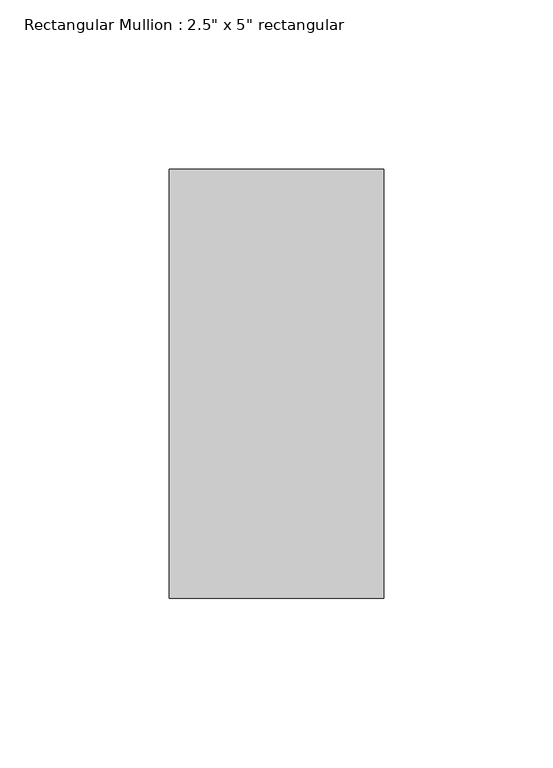
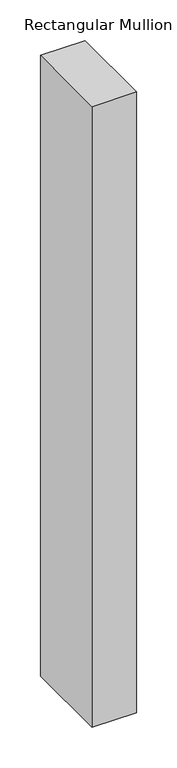
"""IFC4 building model written with IfcOpenShell, lengths in millimetres: member geometry."""

from ifc_helpers import new_model, si_unit, frame, origin, place, context, project, spatial, polyline, outline, extrude, source, transform, mapped, element, save


def member_51239652(model_context):
    return source(origin(), model_context, "Body", "SweptSolid", [
        extrude(outline(polyline([(0.0, 63.5), (0.0, -63.5), (-63.5, -63.5), (-63.5, 63.5), (0.0, 63.5)])), frame((0.0, 0.0, -934.0527116), z_axis=(0.0, 0.0, 1.0), x_axis=(1.0, 0.0, 0.0)), (0.0, 0.0, 1.0), 934.0527116),
    ])


if __name__ == "__main__":
    model = new_model("IFC4")
    model_context = context("Model", 3, world=origin())
    ifc_project = project(units=[si_unit("LENGTHUNIT", "METRE", prefix="MILLI")], contexts=[model_context])
    site = spatial("IfcSite", under=ifc_project)
    building = spatial("IfcBuilding", under=site)
    placement = place(None, origin())
    member_shape = member_51239652(model_context)
    element("IfcMember", 1, ObjectType="Rectangular Mullion : 2.5\" x 5\" rectangular", at=placement, inside=building, context=model_context, shape_type="MappedRepresentation", body=[
        mapped(member_shape, transform((0.0, 0.0, 0.0), x_axis=(1.0, 0.0, 0.0), y_axis=(0.0, 1.0, 0.0), z_axis=(0.0, 0.0, 1.0))),
    ])
    save(model, "model.ifc")

# Revit data of these elements
# Type "Rectangular Mullion : 2.5\" x 5\" rectangular"
#   built-in parameter 1007304 = 0.416667 (stored number, unit not read)
#   built-in parameter 1007301 = 0.104167 (stored number, unit not read)
#   built-in parameter 1007300 = 0.104167 (stored number, unit not read)
# Element 1 (IfcMember, "Rectangular Mullion : 2.5\" x 5\" rectangular")
#   Materials on its faces: "WINDOW FRAMING"
# Materials
#   "WINDOW FRAMING": class "Generic", colour RGB 120 120 120, transparency 0, Cost = 0
